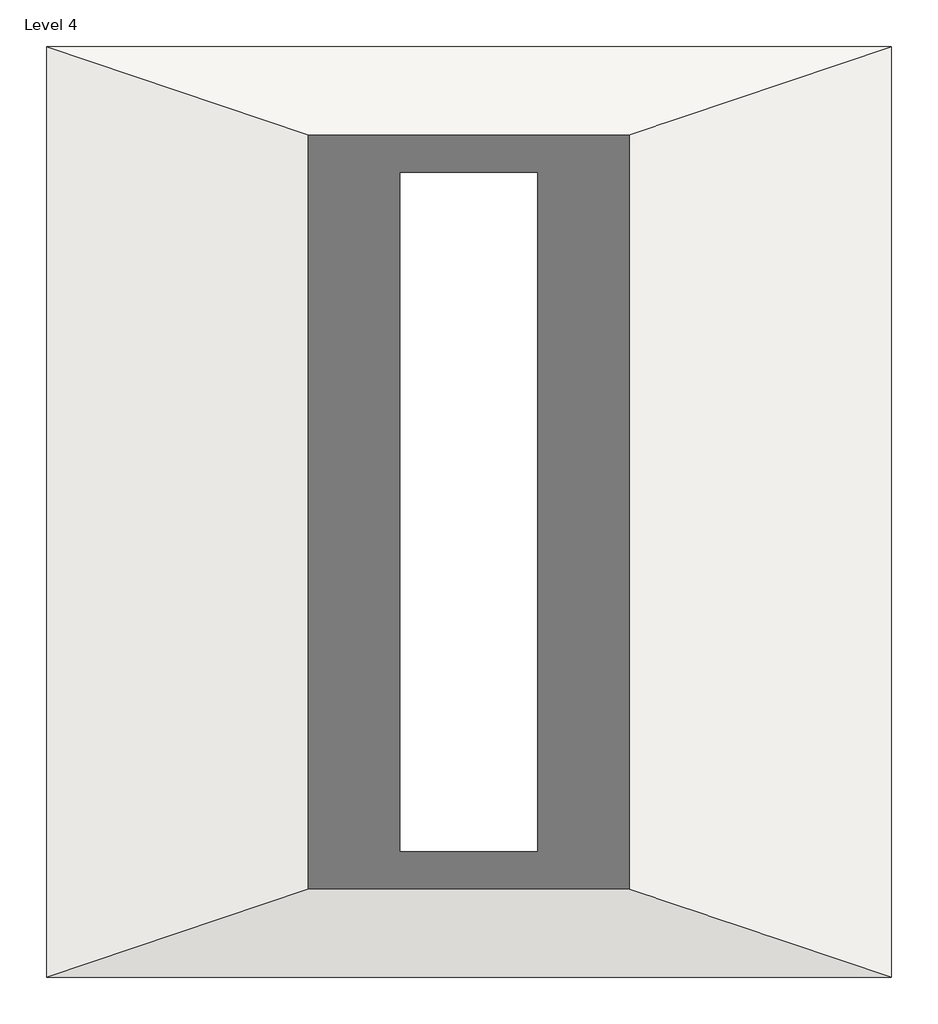
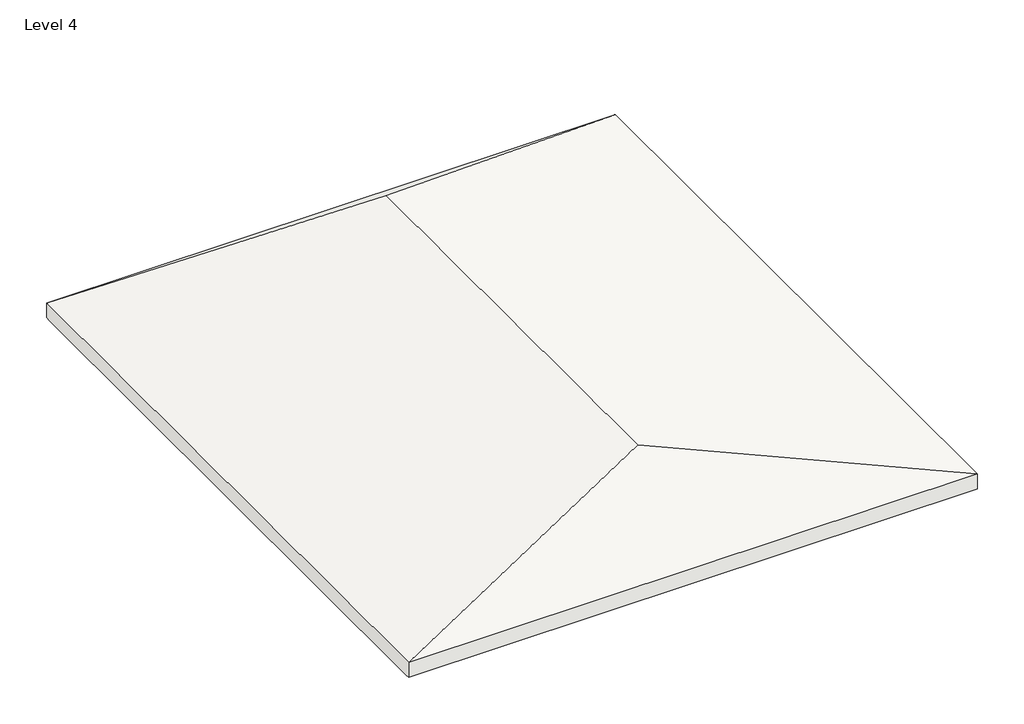
# One storey: 1 roof.
"""IFC4 building model written with IfcOpenShell, lengths in millimetres."""

from ifc_helpers import new_model, si_unit, origin, place, context, project, spatial, faceted_brep, element, save

model = new_model("IFC4")

# Units and contexts
model_context = context("Model", 3, world=origin())
ifc_project = project(units=[si_unit("LENGTHUNIT", "METRE", prefix="MILLI")], contexts=[model_context])

# Site, building, storey
site = spatial("IfcSite", under=ifc_project)
building = spatial("IfcBuilding", under=site)
storey = spatial("IfcBuildingStorey", under=building, Name="Level 4", Elevation=6248.4)

# Roof
placement = place(None, origin())
element("IfcRoof", 1, ObjectType="Generic - 12\"", at=placement, inside=storey, context=model_context, shape_type="Brep", body=[
    faceted_brep([(-11519.7731107, 4047.8631332, 7680.3733136), (-17177.6231107, 5957.1608847, 6248.4), (-5861.9231107, 5957.1608847, 6248.4), (-5861.9231107, -6336.6678486, 6248.4), (-11519.7731107, -4427.3700971, 7680.3733136), (-17177.6231107, -6336.6678486, 6248.4), (-17177.6231107, 6045.9465181, 6562.810775), (-11519.7731107, 4136.6487665, 7994.7840887), (-5861.9231107, 6045.9465181, 6562.810775), (-5861.9231107, -6425.4534819, 6562.810775), (-11519.7731107, -4516.1557304, 7994.7840887), (-17177.6231107, -6425.4534819, 6562.810775), (-17177.6231107, -6425.4534819, 6248.4), (-17177.6231107, 6045.9465181, 6248.4), (-5861.9231107, -6425.4534819, 6248.4), (-5861.9231107, 6045.9465181, 6248.4)], [[[0, 1, 2]], [[3, 4, 0, 2]], [[5, 4, 3]], [[1, 0, 4, 5]], [[6, 7, 8]], [[9, 8, 7, 10]], [[11, 9, 10]], [[6, 11, 10, 7]], [[12, 11, 6, 13, 1, 5]], [[14, 9, 11, 12]], [[15, 8, 9, 14, 3, 2]], [[13, 6, 8, 15]], [[13, 15, 2, 1]], [[3, 14, 12, 5]]]),
])

save(model, "model.ifc")

# Revit data of these elements
# Type "Generic - 12\""
#   Assembly Code = "B1020"
#   Layers, outside or top first: 1' - 0" no material (function 1)
# Element 1 (IfcRoof, "Generic - 12\"")
#   built-in parameter 1001705 = 26.2296 (stored number, unit not read)
#   built-in parameter 1001710 = 33615
#   Phase Created = New Construction
#   Materials on its faces: "Default Roof"
# Materials
#   "Default Roof": colour RGB 88 101 114, transparency 0, Cost = 0
